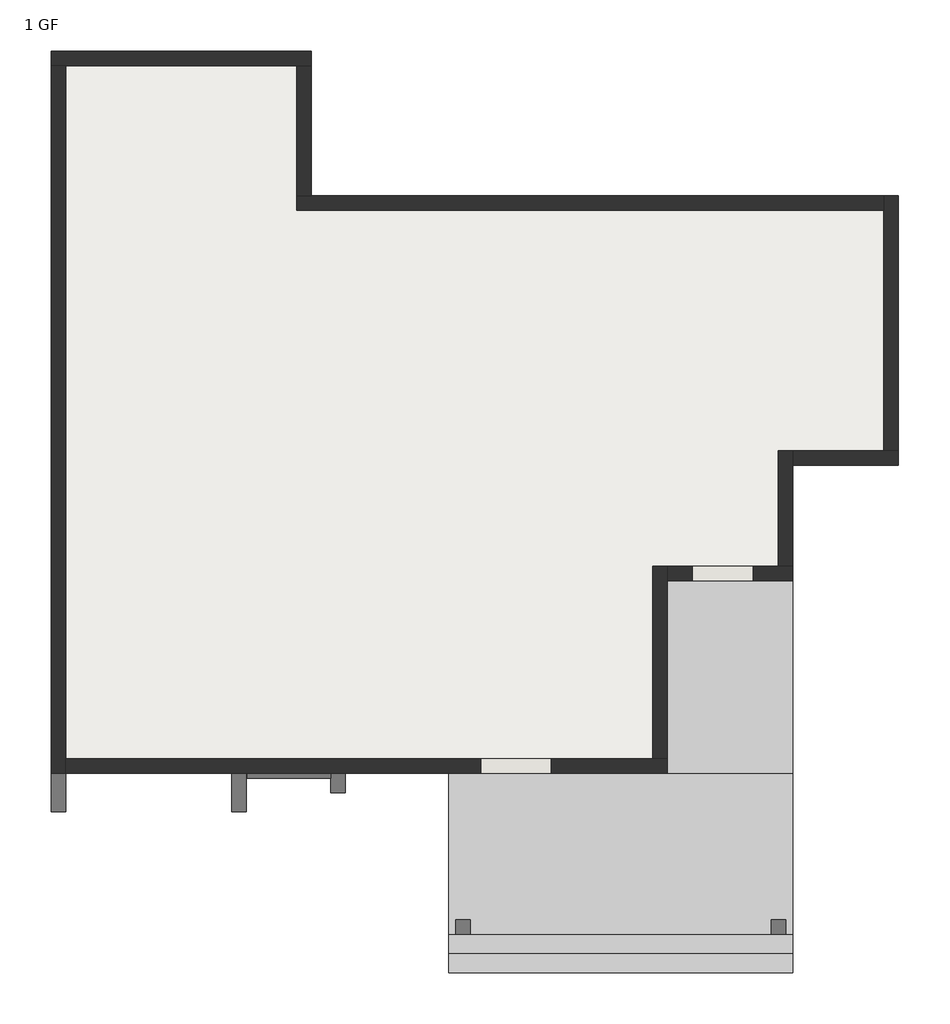
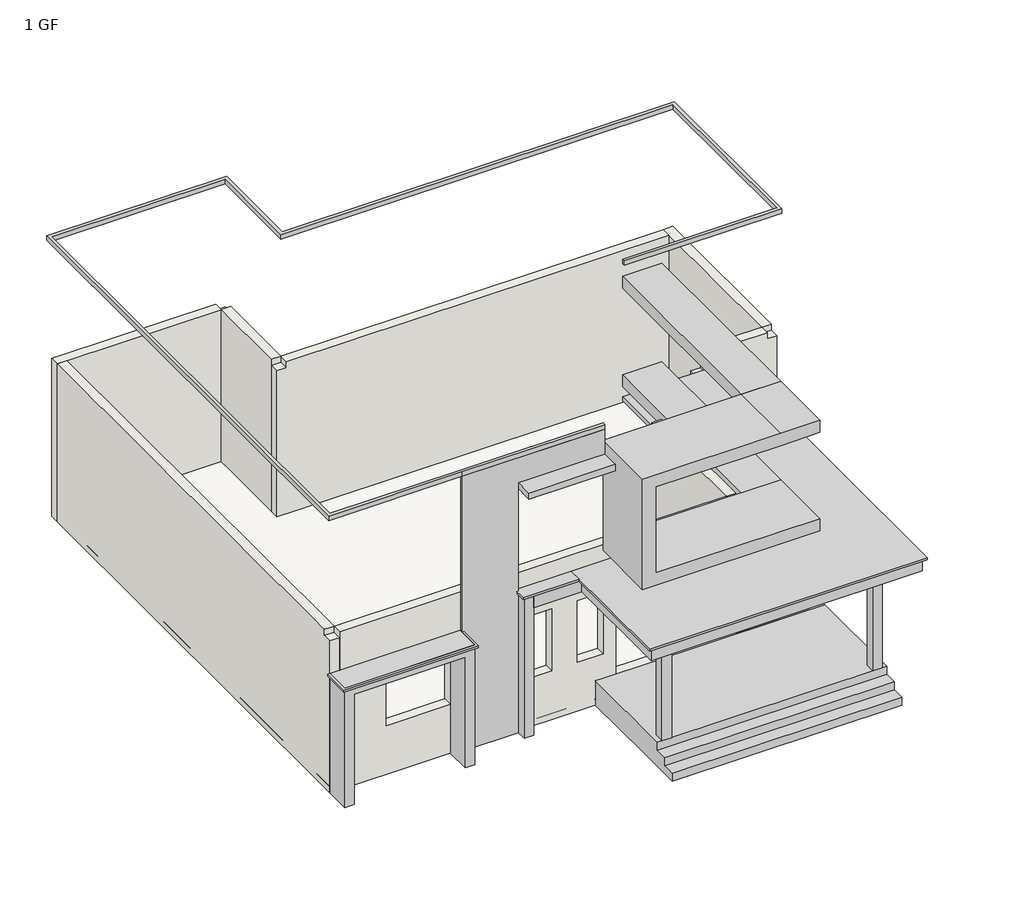
# One storey: 10 walls, 1 proxy, 1 slab.
"""IFC4 building model written with IfcOpenShell, lengths in millimetres."""

from ifc_helpers import new_model, si_unit, origin, origin_with_axes, place, context, project, spatial, polyline, outline, extrude, faceted_brep, transform, mapped, element, save
from components import generic_models_1_generic_models_1_b5997160

model = new_model("IFC4")

# Units and contexts
model_context = context("Model", 3, world=origin())
ifc_project = project(units=[si_unit("LENGTHUNIT", "METRE", prefix="MILLI")], contexts=[model_context])

# Site, building, storey
site = spatial("IfcSite", under=ifc_project)
building = spatial("IfcBuilding", under=site)
storey = spatial("IfcBuildingStorey", under=building, Name="1 GF", Elevation=0.0)

# Proxy
placement = place(None, origin())
generic_models_1_generic_models_1_shape = generic_models_1_generic_models_1_b5997160(model_context)
element("IfcBuildingElementProxy", 1, Name="Generic Models 1 : Generic Models 1", ObjectType="Generic Models 1 : Generic Models 1", at=placement, inside=storey, context=model_context, shape_type="MappedRepresentation", body=[
    mapped(generic_models_1_generic_models_1_shape, transform((0.0, 0.0, 0.0), x_axis=(1.0, 0.0, 0.0), y_axis=(0.0, 1.0, 0.0), z_axis=(0.0, 0.0, 1.0))),
])

# Slab
element("IfcSlab", 2, ObjectType="6\"", at=placement, inside=storey, context=model_context, shape_type="SweptSolid", body=[
    extrude(outline(polyline([(-4260.6149535, 9951.3658196), (-145.8149535, 9951.3658196), (-145.8149535, 7665.3658196), (9150.5850465, 7665.3658196), (9150.5850465, 3398.1658196), (7474.1850465, 3398.1658196), (7474.1850465, 1569.3658196), (5492.9850465, 1569.3658196), (5492.9850465, -1478.6341804), (-4260.6149535, -1478.6341804), (-4260.6149535, 9951.3658196)])), origin_with_axes(), (0.0, 0.0, 1.0), 152.4),
])

# Walls
element("IfcWall", 3, ObjectType="9\" wall", at=placement, inside=storey, context=model_context, shape_type="Brep", body=[
    faceted_brep([(-145.8149535, 9951.3658196, 0.0), (-4260.6149535, 9951.3658196, 0.0), (-4260.6149535, 9951.3658196, 3962.4), (-4032.0149535, 9951.3658196, 3962.4), (-374.4149535, 9951.3658196, 3962.4), (-374.4149535, 9951.3658196, 3810.0), (-145.8149535, 9951.3658196, 3810.0), (-145.8149535, 9722.7658196, 0.0), (-145.8149535, 9722.7658196, 3810.0), (-374.4149535, 9722.7658196, 3810.0), (-374.4149535, 9722.7658196, 3962.4), (-4032.0149535, 9722.7658196, 3962.4), (-4260.6149535, 9722.7658196, 3962.4), (-4260.6149535, 9722.7658196, 0.0), (-4032.0149535, 9722.7658196, 0.0), (-374.4149535, 9722.7658196, 0.0)], [[[0, 1, 2, 3, 4, 5, 6]], [[7, 8, 9, 10, 11, 12, 13, 14, 15]], [[1, 0, 7, 15, 14, 13]], [[4, 3, 2, 12, 11, 10]], [[5, 9, 8, 6]], [[0, 6, 8, 7]], [[5, 4, 10, 9]], [[2, 1, 13, 12]]]),
])
element("IfcWall", 4, ObjectType="9\" wall", at=placement, inside=storey, context=model_context, shape_type="Brep", body=[
    faceted_brep([(-4260.6149535, 9722.7658196, 0.0), (-4260.6149535, -1478.6341804, 0.0), (-4260.6149535, -1478.6341804, 3810.0), (-4260.6149535, -1250.0341804, 3810.0), (-4260.6149535, -1250.0341804, 3962.4), (-4260.6149535, 9722.7658196, 3962.4), (-4032.0149535, 9722.7658196, 0.0), (-4032.0149535, 9722.7658196, 3962.4), (-4032.0149535, -1250.0341804, 3962.4), (-4032.0149535, -1250.0341804, 3810.0), (-4032.0149535, -1478.6341804, 3810.0), (-4032.0149535, -1478.6341804, 0.0), (-4032.0149535, -1250.0341804, 0.0)], [[[0, 1, 2, 3, 4, 5]], [[6, 7, 8, 9, 10, 11, 12]], [[1, 0, 6, 12, 11]], [[5, 4, 8, 7]], [[9, 3, 2, 10]], [[2, 1, 11, 10]], [[4, 3, 9, 8]], [[0, 5, 7, 6]]]),
])
element("IfcWall", 5, ObjectType="9\" wall", at=placement, inside=storey, context=model_context, shape_type="Brep", body=[
    faceted_brep([(-4032.0149535, -1478.6341804, 0.0), (5492.9850465, -1478.6341804, 0.0), (5492.9850465, -1478.6341804, 3810.0), (5264.3850465, -1478.6341804, 3810.0), (5264.3850465, -1478.6341804, 3962.4), (-4032.0149535, -1478.6341804, 3962.4), (-4032.0149535, -1478.6341804, 3810.0), (2533.8850465, -1478.6341804, 609.6), (2533.8850465, -1478.6341804, 2768.6), (3651.4850465, -1478.6341804, 2768.6), (3651.4850465, -1478.6341804, 609.6), (393.9350465, -1478.6341804, 1219.2), (393.9350465, -1478.6341804, 2768.6), (1003.5350465, -1478.6341804, 2768.6), (1003.5350465, -1478.6341804, 1219.2), (2216.3850465, -1478.6341804, 2768.6), (2216.3850465, -1478.6341804, 1219.2), (1606.7850465, -1478.6341804, 1219.2), (1606.7850465, -1478.6341804, 2768.6), (-2927.1149535, -1478.6341804, 1219.2), (-2927.1149535, -1478.6341804, 2768.6), (-1403.1149535, -1478.6341804, 2768.6), (-1403.1149535, -1478.6341804, 1219.2), (3880.0850465, -1478.6341804, 1219.2), (3880.0850465, -1478.6341804, 2768.6), (5099.2850465, -1478.6341804, 2768.6), (5099.2850465, -1478.6341804, 1219.2), (5492.9850465, -1250.0341804, 0.0), (5264.3850465, -1250.0341804, 0.0), (-4032.0149535, -1250.0341804, 0.0), (-4032.0149535, -1250.0341804, 3962.4), (127.2350465, -1250.0341804, 3962.4), (355.8350465, -1250.0341804, 3962.4), (2305.2850465, -1250.0341804, 3962.4), (2533.8850465, -1250.0341804, 3962.4), (5264.3850465, -1250.0341804, 3962.4), (5264.3850465, -1250.0341804, 3810.0), (5492.9850465, -1250.0341804, 3810.0), (2533.8850465, -1250.0341804, 2768.6), (2533.8850465, -1250.0341804, 609.6), (3651.4850465, -1250.0341804, 609.6), (3651.4850465, -1250.0341804, 2768.6), (393.9350465, -1250.0341804, 2768.6), (393.9350465, -1250.0341804, 1219.2), (1003.5350465, -1250.0341804, 1219.2), (1003.5350465, -1250.0341804, 2768.6), (2216.3850465, -1250.0341804, 1219.2), (2216.3850465, -1250.0341804, 2768.6), (1606.7850465, -1250.0341804, 2768.6), (1606.7850465, -1250.0341804, 1219.2), (-2927.1149535, -1250.0341804, 2768.6), (-2927.1149535, -1250.0341804, 1219.2), (-1403.1149535, -1250.0341804, 1219.2), (-1403.1149535, -1250.0341804, 2768.6), (3880.0850465, -1250.0341804, 2768.6), (3880.0850465, -1250.0341804, 1219.2), (5099.2850465, -1250.0341804, 1219.2), (5099.2850465, -1250.0341804, 2768.6)], [[[0, 1, 2, 3, 4, 5, 6], [7, 8, 9, 10], [11, 12, 13, 14], [15, 16, 17, 18], [19, 20, 21, 22], [23, 24, 25, 26]], [[27, 28, 29, 30, 31, 32, 33, 34, 35, 36, 37], [38, 39, 40, 41], [42, 43, 44, 45], [46, 47, 48, 49], [50, 51, 52, 53], [54, 55, 56, 57]], [[1, 0, 29, 28, 27]], [[5, 4, 35, 34, 33, 32, 31, 30]], [[8, 7, 39, 38]], [[9, 8, 38, 41]], [[10, 9, 41, 40]], [[7, 10, 40, 39]], [[11, 43, 42, 12]], [[12, 42, 45, 13]], [[13, 45, 44, 14]], [[43, 11, 14, 44]], [[15, 47, 46, 16]], [[47, 15, 18, 48]], [[48, 18, 17, 49]], [[16, 46, 49, 17]], [[50, 20, 19, 51]], [[20, 50, 53, 21]], [[21, 53, 52, 22]], [[51, 19, 22, 52]], [[29, 0, 6, 5, 30]], [[3, 2, 37, 36]], [[2, 1, 27, 37]], [[4, 3, 36, 35]], [[54, 24, 23, 55]], [[24, 54, 57, 25]], [[25, 57, 56, 26]], [[55, 23, 26, 56]]]),
])
element("IfcWall", 6, ObjectType="9\" wall", at=placement, inside=storey, context=model_context, shape_type="Brep", body=[
    faceted_brep([(5492.9850465, -1250.0341804, 3962.4), (5492.9850465, -1250.0341804, 3810.0), (5492.9850465, -1250.0341804, 0.0), (5492.9850465, 1569.3658196, 0.0), (5492.9850465, 1797.9658196, 0.0), (5492.9850465, 1797.9658196, 3457.4791506), (5492.9850465, 1797.9658196, 3962.4), (5264.3850465, -1250.0341804, 0.0), (5264.3850465, -1250.0341804, 3962.4), (5264.3850465, 1797.9658196, 3962.4), (5264.3850465, 1797.9658196, 0.0)], [[[0, 1, 2, 3, 4, 5, 6]], [[7, 8, 9, 10]], [[4, 3, 2, 7, 10]], [[0, 6, 9, 8]], [[6, 5, 4, 10, 9]], [[0, 8, 7, 2, 1]]]),
])
element("IfcWall", 7, ObjectType="9\" wall", at=placement, inside=storey, context=model_context, shape_type="Brep", body=[
    faceted_brep([(5492.9850465, 1569.3658196, 0.0), (7474.1850465, 1569.3658196, 0.0), (7474.1850465, 1569.3658196, 3457.4791506), (5492.9850465, 1569.3658196, 3457.4791506), (6851.8850465, 1569.3658196, 609.6), (5886.6850465, 1569.3658196, 609.6), (5886.6850465, 1569.3658196, 2768.6), (6851.8850465, 1569.3658196, 2768.6), (5492.9850465, 1797.9658196, 0.0), (5492.9850465, 1797.9658196, 3457.4791506), (7245.5850465, 1797.9658196, 3457.4791506), (7474.1850465, 1797.9658196, 3457.4791506), (7474.1850465, 1797.9658196, 0.0), (7245.5850465, 1797.9658196, 0.0), (6851.8850465, 1797.9658196, 609.6), (6851.8850465, 1797.9658196, 2768.6), (5886.6850465, 1797.9658196, 2768.6), (5886.6850465, 1797.9658196, 609.6)], [[[0, 1, 2, 3], [4, 5, 6, 7]], [[8, 9, 10, 11, 12, 13], [14, 15, 16, 17]], [[1, 0, 8, 13, 12]], [[3, 2, 11, 10, 9]], [[0, 3, 9, 8]], [[2, 1, 12, 11]], [[15, 14, 4, 7]], [[16, 15, 7, 6]], [[17, 16, 6, 5]], [[14, 17, 5, 4]]]),
])
element("IfcWall", 8, ObjectType="9\" wall", at=placement, inside=storey, context=model_context, shape_type="Brep", body=[
    faceted_brep([(7474.1850465, 1797.9658196, 0.0), (7474.1850465, 3398.1658196, 0.0), (7474.1850465, 3626.7658196, 0.0), (7474.1850465, 3626.7658196, 3457.4791506), (7474.1850465, 1797.9658196, 3457.4791506), (7245.5850465, 1797.9658196, 0.0), (7245.5850465, 1797.9658196, 3457.4791506), (7245.5850465, 3626.7658196, 3457.4791506), (7245.5850465, 3626.7658196, 0.0)], [[[0, 1, 2, 3, 4]], [[5, 6, 7, 8]], [[2, 1, 0, 5, 8]], [[4, 3, 7, 6]], [[0, 4, 6, 5]], [[3, 2, 8, 7]]]),
])
element("IfcWall", 9, ObjectType="9\" wall", at=placement, inside=storey, context=model_context, shape_type="Brep", body=[
    faceted_brep([(7474.1850465, 3398.1658196, 0.0), (9150.5850465, 3398.1658196, 0.0), (9150.5850465, 3398.1658196, 3810.0), (8921.9850465, 3398.1658196, 3810.0), (8921.9850465, 3398.1658196, 3962.4), (7474.1850465, 3398.1658196, 3962.4), (7474.1850465, 3626.7658196, 0.0), (7474.1850465, 3626.7658196, 3457.4791506), (7474.1850465, 3626.7658196, 3962.4), (8921.9850465, 3626.7658196, 3962.4), (8921.9850465, 3626.7658196, 3810.0), (9150.5850465, 3626.7658196, 3810.0), (9150.5850465, 3626.7658196, 0.0), (8921.9850465, 3626.7658196, 0.0)], [[[0, 1, 2, 3, 4, 5]], [[6, 7, 8, 9, 10, 11, 12, 13]], [[1, 0, 6, 13, 12]], [[5, 4, 9, 8]], [[0, 5, 8, 7, 6]], [[10, 3, 2, 11]], [[2, 1, 12, 11]], [[4, 3, 10, 9]]]),
])
element("IfcWall", 10, ObjectType="9\" wall", at=placement, inside=storey, context=model_context, shape_type="Brep", body=[
    faceted_brep([(9150.5850465, 3626.7658196, 3962.4), (9150.5850465, 3626.7658196, 3810.0), (9150.5850465, 3626.7658196, 0.0), (9150.5850465, 7665.3658196, 0.0), (9150.5850465, 7665.3658196, 3962.4), (9150.5850465, 7436.7658196, 3962.4), (8921.9850465, 3626.7658196, 0.0), (8921.9850465, 3626.7658196, 3962.4), (8921.9850465, 7436.7658196, 3962.4), (8921.9850465, 7665.3658196, 3962.4), (8921.9850465, 7665.3658196, 0.0), (8921.9850465, 7436.7658196, 0.0)], [[[0, 1, 2, 3, 4, 5]], [[6, 7, 8, 9, 10, 11]], [[3, 2, 6, 11, 10]], [[0, 5, 4, 9, 8, 7]], [[3, 10, 9, 4]], [[0, 7, 6, 2, 1]]]),
])
element("IfcWall", 11, ObjectType="9\" wall", at=placement, inside=storey, context=model_context, shape_type="Brep", body=[
    faceted_brep([(8921.9850465, 7665.3658196, 3962.4), (8921.9850465, 7665.3658196, 3810.0), (8921.9850465, 7665.3658196, 0.0), (-145.8149535, 7665.3658196, 0.0), (-374.4149535, 7665.3658196, 0.0), (-374.4149535, 7665.3658196, 3810.0), (-145.8149535, 7665.3658196, 3810.0), (-145.8149535, 7665.3658196, 3962.4), (8921.9850465, 7436.7658196, 0.0), (8921.9850465, 7436.7658196, 3962.4), (-145.8149535, 7436.7658196, 3962.4), (-145.8149535, 7436.7658196, 3810.0), (-374.4149535, 7436.7658196, 3810.0), (-374.4149535, 7436.7658196, 0.0)], [[[0, 1, 2, 3, 4, 5, 6, 7]], [[8, 9, 10, 11, 12, 13]], [[4, 3, 2, 8, 13]], [[0, 7, 10, 9]], [[11, 6, 5, 12]], [[5, 4, 13, 12]], [[7, 6, 11, 10]], [[0, 9, 8, 2, 1]]]),
])
element("IfcWall", 12, ObjectType="9\" wall", at=placement, inside=storey, context=model_context, shape_type="Brep", body=[
    faceted_brep([(-145.8149535, 7665.3658196, 3962.4), (-145.8149535, 7665.3658196, 0.0), (-145.8149535, 9722.7658196, 0.0), (-145.8149535, 9722.7658196, 3810.0), (-145.8149535, 9722.7658196, 3962.4), (-374.4149535, 7665.3658196, 0.0), (-374.4149535, 7665.3658196, 3810.0), (-374.4149535, 7665.3658196, 3962.4), (-374.4149535, 9722.7658196, 3962.4), (-374.4149535, 9722.7658196, 0.0)], [[[0, 1, 2, 3, 4]], [[5, 6, 7, 8, 9]], [[2, 1, 5, 9]], [[0, 4, 8, 7]], [[2, 9, 8, 4, 3]], [[0, 7, 6, 5, 1]]]),
])

save(model, "model.ifc")

# Revit data of these elements
# Type "6\""
#   Assembly Code = "B1010"
#   Function = 0
#   Layers, outside or top first: 0' - 6" no material (function 1)
# Type "9\" wall"
#   Assembly Code = "B2010"
#   Layers, outside or top first: 0' - 9" no material (function 1)
# Element 1 (IfcBuildingElementProxy, "Generic Models 1 : Generic Models 1")
#   Phase Created = New Construction
# Element 2 (IfcSlab, "6\"")
#   built-in parameter 1001955 = 3.14159 (stored number, unit not read)
#   Height Offset From Level = 0' - 6"
#   Phase Created = New Construction
#   Materials on its faces: "Default Floor"
# Elements 3, 4, 5, 6, 9, 10, 11, 12 (IfcWall, "9\" wall")
#   Top Offset = 0' - 0"
#   Base Offset = 0' - 0"
#   wall height = 13' - 0"
#   Phase Created = New Construction
#   Base Constraint = 1 GF
#   Top Constraint = 3 SLAB
#   Materials on its faces: "Default Wall"
# Elements 7, 8 (IfcWall, "9\" wall")
#   Top Offset = -1' - 7.87877"
#   Base Offset = 0' - 0"
#   wall height = 11' - 4.12123"
#   Phase Created = New Construction
#   Base Constraint = 1 GF
#   Top Constraint = 3 SLAB
#   Materials on its faces: "Default Wall"
# Materials
#   "Default Floor": colour RGB 128 128 128, transparency 0, Cost = 0
#   "Default Wall": colour RGB 128 128 128, transparency 0, Cost = 0
